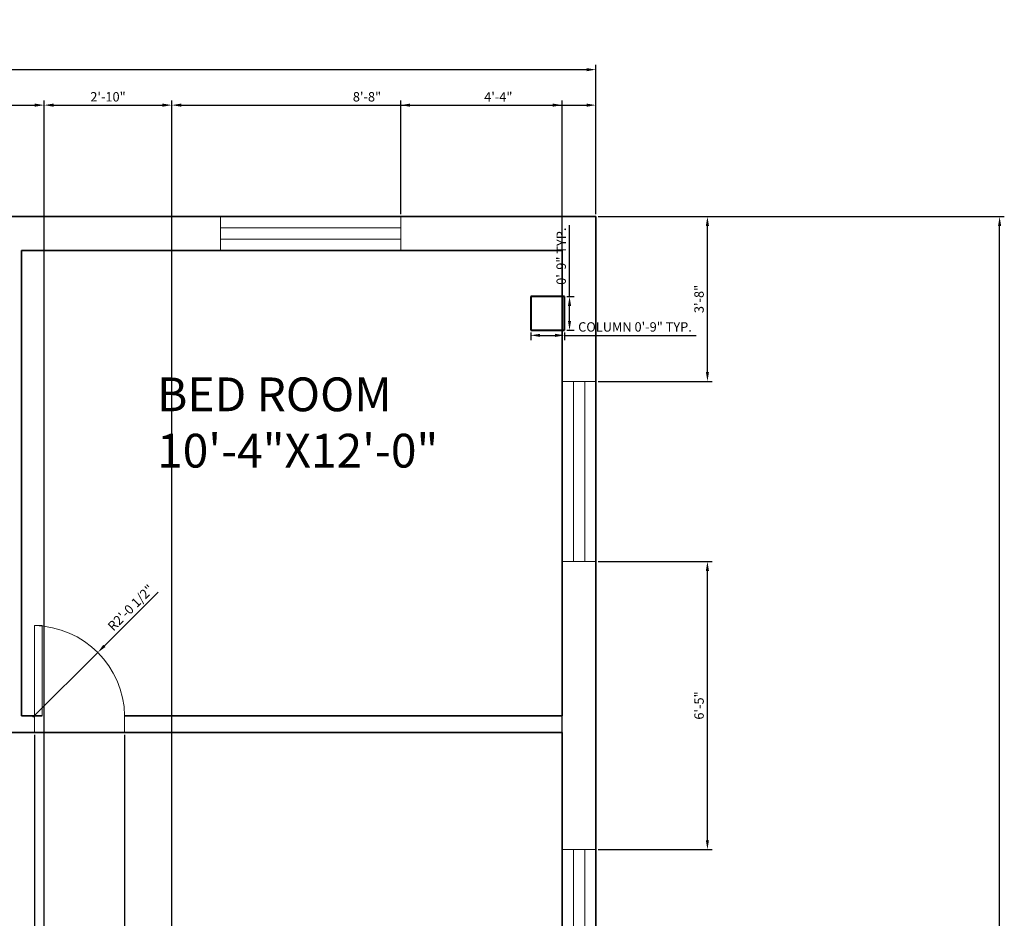
# Model space of a CAD drawing. Units: millimetres. Extents: x 2124 to 2653, y 1244 to 1836.
# Tile 4 of 4: x 2390 to 2653, y 1597 to 1836. Entities that reach past the tile are written whole.
import ezdxf

# ---------------------------------------------------------------- set-up
doc = ezdxf.new("R2010")
doc.units = ezdxf.units.MM
for name, color, linetype, lineweight in [('A-ANNO-DIMS', 2, 'Continuous', 18), ('A-AREA-IDEN', 7, 'Continuous', 18), ('A-COLS', 1, 'Continuous', 40), ('A-DOOR', 3, 'Continuous', 18), ('A-GLAZ', 4, 'Continuous', 18), ('A-WALL', 7, 'Continuous', 35)]:
    doc.layers.add(name, color=color, linetype=linetype, lineweight=lineweight)
doc.styles.get("Standard").update_dxf_attribs({"font": 'arial.ttf'})
doc.dimstyles.new('ISO-25', dxfattribs={"dimtxt": 2.5, "dimasz": 2.5, "dimexe": 1.25, "dimexo": 0.625, "dimtad": 1, "dimdec": 0, "dimlunit": 3, "dimtxsty": 'Standard', "dimcen": 2.5, "dimadec": 0, "dimazin": 0, "dimtfac": 1, "dimtdec": 0, "dimtmove": 0, "dimatfit": 3, "dimfxl": 1, "dimarcsym": 0})

# ---------------------------------------------------------------- blocks, each defined once
blk = doc.blocks.new('*D8')
at = {"layer": 'A-ANNO-DIMS', "color": 0, "lineweight": -2, "transparency": 16777216}
for p, q in [((2159.76, 1784.37), (2159.76, 1824.15)), ((2162.26, 1822.9), (2541.26, 1822.9)), ((2543.76, 1784.37), (2543.76, 1824.15))]:
    blk.add_line(p, q, dxfattribs=at)
at = {"layer": 'A-ANNO-DIMS', "color": 0, "transparency": 16777216}
for points in [[(2162.26, 1823.31), (2162.26, 1822.48), (2159.76, 1822.9)], [(2541.26, 1823.31), (2541.26, 1822.48), (2543.76, 1822.9)]]:
    blk.add_solid(points, dxfattribs=at)
at = {"layer": 'Defpoints', "color": 0, "transparency": 16777216}
for p in [(2543.76, 1822.9), (2159.76, 1783.74), (2543.76, 1783.74)]:
    blk.add_point(p, dxfattribs=at)
at = {"layer": 'A-ANNO-DIMS', "color": 0, "transparency": 16777216, "insert": (2351.76, 1829.59), "char_height": 2.5, "attachment_point": 5}
blk.add_mtext("{\\fCambria|b0|i0|c0|p18;\\H4.8x;32'}", dxfattribs=at)
blk = doc.blocks.new('*D9')
at = {"layer": 'A-ANNO-DIMS', "color": 0, "lineweight": -2, "transparency": 16777216}
for p, q in [((2544.38, 1783.74), (2652.54, 1783.74)), ((2651.29, 1289.47), (2651.29, 1781.24)), ((2544.38, 1286.97), (2652.54, 1286.97))]:
    blk.add_line(p, q, dxfattribs=at)
at = {"layer": 'A-ANNO-DIMS', "color": 0, "transparency": 16777216}
for points in [[(2650.87, 1781.24), (2651.71, 1781.24), (2651.29, 1783.74)], [(2650.87, 1289.47), (2651.71, 1289.47), (2651.29, 1286.97)]]:
    blk.add_solid(points, dxfattribs=at)
at = {"layer": 'Defpoints', "color": 0, "transparency": 16777216}
for p in [(2543.76, 1783.74), (2651.29, 1783.74), (2543.76, 1286.97)]:
    blk.add_point(p, dxfattribs=at)
at = {"layer": 'A-ANNO-DIMS', "color": 0, "transparency": 16777216, "insert": (2644.38, 1535.36), "char_height": 2.5, "width": 21.1968, "attachment_point": 5, "rotation": 90}
blk.add_mtext('{\\fCambria|b0|i0|c0|p18;\\H4.8x;45\'-0"}', dxfattribs=at)
blk = doc.blocks.new('WINDOW-4FT')
for p, q in [((48, 9), (0, 9)), ((0, 9), (0, 0)), ((48, 0), (48, 9)), ((48, 6), (0, 6)), ((48, 3), (0, 3)), ((0, 0), (48, 0))]:
    blk.add_line(p, q)
blk = doc.blocks.new('WINDOW-2FT')
for p, q in [((9, 24), (0, 24)), ((0, 24), (0, 0)), ((3, 0), (3, 24)), ((6, 0), (6, 24)), ((9, 0), (9, 24)), ((0, 0), (9, 0))]:
    blk.add_line(p, q)
blk = doc.blocks.new('COLUMN-9IN-SQ')
for p, q in [((9, 9), (0, 9)), ((0, 9), (0, 0)), ((9, 0), (9, 9)), ((0, 0), (9, 0))]:
    blk.add_line(p, q)
blk = doc.blocks.new('*D16')
at = {"layer": 'A-ANNO-DIMS', "color": 0, "lineweight": -2, "transparency": 16777216}
for p, q in [((2526.38, 1752.82), (2526.38, 1750.85)), ((2528.88, 1752.1), (2532.88, 1752.1)), ((2535.38, 1752.82), (2535.38, 1750.85)), ((2535.38, 1752.1), (2570.44, 1752.1))]:
    blk.add_line(p, q, dxfattribs=at)
at = {"layer": 'A-ANNO-DIMS', "color": 0, "transparency": 16777216}
for points in [[(2528.88, 1752.51), (2528.88, 1751.68), (2526.38, 1752.1)], [(2532.88, 1752.51), (2532.88, 1751.68), (2535.38, 1752.1)]]:
    blk.add_solid(points, dxfattribs=at)
at = {"layer": 'Defpoints', "color": 0, "transparency": 16777216}
for p in [(2526.38, 1753.45), (2535.38, 1753.45), (2535.38, 1752.1)]:
    blk.add_point(p, dxfattribs=at)
at = {"layer": 'A-ANNO-DIMS', "color": 0, "transparency": 16777216, "insert": (2554.16, 1754.02), "char_height": 2.5, "attachment_point": 5}
blk.add_mtext('COLUMN 0\'-9" TYP.', dxfattribs=at)
blk = doc.blocks.new('*D17')
at = {"layer": 'A-ANNO-DIMS', "color": 0, "lineweight": -2, "transparency": 16777216}
for p, q in [((2536.73, 1762.45), (2536.73, 1781.44)), ((2536, 1762.45), (2537.98, 1762.45)), ((2536.73, 1755.95), (2536.73, 1759.95)), ((2536, 1753.45), (2537.98, 1753.45))]:
    blk.add_line(p, q, dxfattribs=at)
at = {"layer": 'A-ANNO-DIMS', "color": 0, "transparency": 16777216}
for points in [[(2536.31, 1759.95), (2537.14, 1759.95), (2536.73, 1762.45)], [(2536.31, 1755.95), (2537.14, 1755.95), (2536.73, 1753.45)]]:
    blk.add_solid(points, dxfattribs=at)
at = {"layer": 'Defpoints', "color": 0, "transparency": 16777216}
for p in [(2535.38, 1762.45), (2536.73, 1762.45), (2535.38, 1753.45)]:
    blk.add_point(p, dxfattribs=at)
at = {"layer": 'A-ANNO-DIMS', "color": 0, "transparency": 16777216, "insert": (2534.83, 1773.19), "char_height": 2.5, "attachment_point": 5, "rotation": 90}
blk.add_mtext('0\'-9" TYP.', dxfattribs=at)
blk = doc.blocks.new('*D22')
at = {"layer": 'A-ANNO-DIMS', "color": 0, "lineweight": -2, "transparency": 16777216}
for p, q in [((2491.76, 1784.37), (2491.76, 1814.69)), ((2494.26, 1813.44), (2541.26, 1813.44)), ((2543.76, 1784.37), (2543.76, 1814.69))]:
    blk.add_line(p, q, dxfattribs=at)
at = {"layer": 'A-ANNO-DIMS', "color": 0, "transparency": 16777216}
for points in [[(2494.26, 1813.86), (2494.26, 1813.02), (2491.76, 1813.44)], [(2541.26, 1813.86), (2541.26, 1813.02), (2543.76, 1813.44)]]:
    blk.add_solid(points, dxfattribs=at)
at = {"layer": 'Defpoints', "color": 0, "transparency": 16777216}
for p in [(2543.76, 1813.44), (2491.76, 1783.74), (2543.76, 1783.74)]:
    blk.add_point(p, dxfattribs=at)
at = {"layer": 'A-ANNO-DIMS', "color": 0, "transparency": 16777216, "insert": (2517.76, 1815.32), "char_height": 2.5, "attachment_point": 5}
blk.add_mtext('4\'-4"', dxfattribs=at)
blk = doc.blocks.new('*D24')
at = {"layer": 'A-ANNO-DIMS', "color": 0, "lineweight": -2, "transparency": 16777216}
for p, q in [((2544.38, 1783.74), (2574.71, 1783.74)), ((2573.46, 1742.34), (2573.46, 1781.24)), ((2544.38, 1739.84), (2574.71, 1739.84))]:
    blk.add_line(p, q, dxfattribs=at)
at = {"layer": 'A-ANNO-DIMS', "color": 0, "transparency": 16777216}
for points in [[(2573.04, 1781.24), (2573.87, 1781.24), (2573.46, 1783.74)], [(2573.04, 1742.34), (2573.87, 1742.34), (2573.46, 1739.84)]]:
    blk.add_solid(points, dxfattribs=at)
at = {"layer": 'Defpoints', "color": 0, "transparency": 16777216}
for p in [(2543.76, 1783.74), (2573.46, 1783.74), (2543.76, 1739.84)]:
    blk.add_point(p, dxfattribs=at)
at = {"layer": 'A-ANNO-DIMS', "color": 0, "transparency": 16777216, "insert": (2571.55, 1761.79), "char_height": 2.5, "attachment_point": 5, "rotation": 90}
blk.add_mtext('3\'-8"', dxfattribs=at)
blk = doc.blocks.new('*D25')
at = {"layer": 'A-ANNO-DIMS', "color": 0, "lineweight": -2, "transparency": 16777216}
for p, q in [((2544.38, 1691.84), (2574.71, 1691.84)), ((2573.46, 1617.57), (2573.46, 1689.34)), ((2544.38, 1615.07), (2574.71, 1615.07))]:
    blk.add_line(p, q, dxfattribs=at)
at = {"layer": 'A-ANNO-DIMS', "color": 0, "transparency": 16777216}
for points in [[(2573.04, 1689.34), (2573.87, 1689.34), (2573.46, 1691.84)], [(2573.04, 1617.57), (2573.87, 1617.57), (2573.46, 1615.07)]]:
    blk.add_solid(points, dxfattribs=at)
at = {"layer": 'Defpoints', "color": 0, "transparency": 16777216}
for p in [(2543.76, 1691.84), (2573.46, 1691.84), (2543.76, 1615.07)]:
    blk.add_point(p, dxfattribs=at)
at = {"layer": 'A-ANNO-DIMS', "color": 0, "transparency": 16777216, "insert": (2571.55, 1653.46), "char_height": 2.5, "attachment_point": 5, "rotation": 90}
blk.add_mtext('6\'-5"', dxfattribs=at)
blk = doc.blocks.new('*D43')
at = {"layer": 'A-ANNO-DIMS', "color": 0, "lineweight": -2, "transparency": 16777216}
for p, q in [((2383.02, 1645.62), (2383.02, 1256.02)), ((2394.21, 1645.62), (2394.21, 1256.02)), ((2385.52, 1257.27), (2391.71, 1257.27))]:
    blk.add_line(p, q, dxfattribs=at)
at = {"layer": 'A-ANNO-DIMS', "color": 0, "transparency": 16777216}
for points in [[(2385.52, 1257.69), (2385.52, 1256.86), (2383.02, 1257.27)], [(2391.71, 1257.69), (2391.71, 1256.86), (2394.21, 1257.27)]]:
    blk.add_solid(points, dxfattribs=at)
at = {"layer": 'Defpoints', "color": 0, "transparency": 16777216}
for p in [(2383.02, 1646.24), (2394.21, 1646.24), (2394.21, 1257.27)]:
    blk.add_point(p, dxfattribs=at)
at = {"layer": 'A-ANNO-DIMS', "color": 0, "transparency": 16777216, "insert": (2388.62, 1259.18), "char_height": 2.5, "attachment_point": 5}
blk.add_mtext('0\'-11"', dxfattribs=at)
blk = doc.blocks.new('*D44')
at = {"layer": 'A-ANNO-DIMS', "color": 0, "lineweight": -2, "transparency": 16777216}
for p, q in [((2394.21, 1645.62), (2394.21, 1256.02)), ((2418.21, 1645.62), (2418.21, 1256.02)), ((2396.71, 1257.27), (2415.71, 1257.27))]:
    blk.add_line(p, q, dxfattribs=at)
at = {"layer": 'A-ANNO-DIMS', "color": 0, "transparency": 16777216}
for points in [[(2396.71, 1257.69), (2396.71, 1256.86), (2394.21, 1257.27)], [(2415.71, 1257.69), (2415.71, 1256.86), (2418.21, 1257.27)]]:
    blk.add_solid(points, dxfattribs=at)
at = {"layer": 'Defpoints', "color": 0, "transparency": 16777216}
for p in [(2394.21, 1646.24), (2418.21, 1646.24), (2418.21, 1257.27)]:
    blk.add_point(p, dxfattribs=at)
at = {"layer": 'A-ANNO-DIMS', "color": 0, "transparency": 16777216, "insert": (2406.21, 1259.18), "char_height": 2.5, "attachment_point": 5}
blk.add_mtext('2\'-0"', dxfattribs=at)
blk = doc.blocks.new('*D45')
at = {"layer": 'A-ANNO-DIMS', "color": 0, "lineweight": -2, "transparency": 16777216}
for p, q in [((2418.21, 1645.62), (2418.21, 1256.02)), ((2534.76, 1645.62), (2534.76, 1256.02)), ((2420.71, 1257.27), (2532.26, 1257.27))]:
    blk.add_line(p, q, dxfattribs=at)
at = {"layer": 'A-ANNO-DIMS', "color": 0, "transparency": 16777216}
for points in [[(2420.71, 1257.69), (2420.71, 1256.86), (2418.21, 1257.27)], [(2532.26, 1257.69), (2532.26, 1256.86), (2534.76, 1257.27)]]:
    blk.add_solid(points, dxfattribs=at)
at = {"layer": 'Defpoints', "color": 0, "transparency": 16777216}
for p in [(2418.21, 1646.24), (2534.76, 1646.24), (2534.76, 1257.27)]:
    blk.add_point(p, dxfattribs=at)
at = {"layer": 'A-ANNO-DIMS', "color": 0, "transparency": 16777216, "insert": (2476.48, 1259.19), "char_height": 2.5, "attachment_point": 5}
blk.add_mtext('9\'-8 1/2"', dxfattribs=at)
blk = doc.blocks.new('*D47')
at = {"layer": 'A-ANNO-DIMS', "color": 0, "lineweight": -2, "transparency": 16777216}
for p, q in [((2365.24, 1448.87), (2365.24, 1814.69)), ((2367.74, 1813.44), (2394.29, 1813.44)), ((2396.79, 1448.87), (2396.79, 1814.69))]:
    blk.add_line(p, q, dxfattribs=at)
at = {"layer": 'A-ANNO-DIMS', "color": 0, "transparency": 16777216}
for points in [[(2367.74, 1813.86), (2367.74, 1813.02), (2365.24, 1813.44)], [(2394.29, 1813.86), (2394.29, 1813.02), (2396.79, 1813.44)]]:
    blk.add_solid(points, dxfattribs=at)
at = {"layer": 'Defpoints', "color": 0, "transparency": 16777216}
for p in [(2396.79, 1813.44), (2365.24, 1448.24), (2396.79, 1448.24)]:
    blk.add_point(p, dxfattribs=at)
at = {"layer": 'A-ANNO-DIMS', "color": 0, "transparency": 16777216, "insert": (2381.02, 1815.36), "char_height": 2.5, "attachment_point": 5}
blk.add_mtext('2\'-7 1/2"', dxfattribs=at)
blk = doc.blocks.new('*D48')
at = {"layer": 'A-ANNO-DIMS', "color": 0, "lineweight": -2, "transparency": 16777216}
for p, q in [((2396.79, 1448.87), (2396.79, 1814.69)), ((2399.29, 1813.44), (2428.29, 1813.44)), ((2430.79, 1448.87), (2430.79, 1814.69))]:
    blk.add_line(p, q, dxfattribs=at)
at = {"layer": 'A-ANNO-DIMS', "color": 0, "transparency": 16777216}
for points in [[(2399.29, 1813.86), (2399.29, 1813.02), (2396.79, 1813.44)], [(2428.29, 1813.86), (2428.29, 1813.02), (2430.79, 1813.44)]]:
    blk.add_solid(points, dxfattribs=at)
at = {"layer": 'Defpoints', "color": 0, "transparency": 16777216}
for p in [(2430.79, 1813.44), (2396.79, 1448.24), (2430.79, 1448.24)]:
    blk.add_point(p, dxfattribs=at)
at = {"layer": 'A-ANNO-DIMS', "color": 0, "transparency": 16777216, "insert": (2413.79, 1815.34), "char_height": 2.5, "attachment_point": 5}
blk.add_mtext('2\'-10"', dxfattribs=at)
blk = doc.blocks.new('*D49')
at = {"layer": 'A-ANNO-DIMS', "color": 0, "lineweight": -2, "transparency": 16777216}
for p, q in [((2430.79, 1448.87), (2430.79, 1814.69)), ((2433.29, 1813.44), (2532.26, 1813.44)), ((2534.76, 1448.87), (2534.76, 1814.69))]:
    blk.add_line(p, q, dxfattribs=at)
at = {"layer": 'A-ANNO-DIMS', "color": 0, "transparency": 16777216}
for points in [[(2433.29, 1813.86), (2433.29, 1813.02), (2430.79, 1813.44)], [(2532.26, 1813.86), (2532.26, 1813.02), (2534.76, 1813.44)]]:
    blk.add_solid(points, dxfattribs=at)
at = {"layer": 'Defpoints', "color": 0, "transparency": 16777216}
for p in [(2534.76, 1813.44), (2430.79, 1448.24), (2534.76, 1448.24)]:
    blk.add_point(p, dxfattribs=at)
at = {"layer": 'A-ANNO-DIMS', "color": 0, "transparency": 16777216, "insert": (2482.77, 1815.34), "char_height": 2.5, "attachment_point": 5}
blk.add_mtext('8\'-8"', dxfattribs=at)
blk = doc.blocks.new('*D61')
at = {"layer": 'A-ANNO-DIMS', "color": 0, "lineweight": -2, "transparency": 16777216}
for p, q in [((2427.12, 1683.65), (2412.83, 1669.35)), ((2393.78, 1650.31), (2411.06, 1667.59))]:
    blk.add_line(p, q, dxfattribs=at)
at = {"layer": 'A-ANNO-DIMS', "color": 0, "transparency": 16777216}
blk.add_solid([(2412.53, 1669.65), (2413.12, 1669.06), (2411.06, 1667.59)], dxfattribs=at)
at = {"layer": 'Defpoints', "color": 0, "transparency": 16777216}
for p in [(2411.06, 1667.59), (2393.78, 1650.31)]:
    blk.add_point(p, dxfattribs=at)
at = {"layer": 'A-ANNO-DIMS', "color": 0, "transparency": 16777216, "insert": (2420.07, 1679.31), "char_height": 2.5, "attachment_point": 5, "rotation": 44.9997}
blk.add_mtext('R2\'-0 1/2"', dxfattribs=at)

msp = doc.modelspace()

# ---------------------------------------------------------------- linework, layer by layer
at = {"layer": 'A-DOOR'}
for p, q in [((2394.21, 1650.74), (2394.21, 1674.74)), ((2394.21, 1674.74), (2396.21, 1674.74)), ((2396.21, 1674.74), (2396.21, 1650.74)), ((2394.21, 1646.24), (2394.21, 1650.74)), ((2418.21, 1646.24), (2418.21, 1650.74))]:
    msp.add_line(p, q, dxfattribs=at)
msp.add_arc((2393.78, 1650.31), 24.44, 1.016, 88.984, dxfattribs=at)
at = {"layer": 'A-GLAZ'}
msp.add_line((2473.58, 1777.74), (2471.58, 1777.74), dxfattribs=at)
at = {"layer": 'A-WALL'}
for p, q in [((2543.76, 1783.74), (2159.76, 1783.74)), ((2543.76, 1286.97), (2543.76, 1783.74)), ((2534.76, 1774.74), (2390.76, 1774.74)), ((2390.76, 1650.74), (2390.76, 1774.74)), ((2534.76, 1650.74), (2534.76, 1774.74)), ((2396.21, 1650.74), (2390.76, 1650.74)), ((2534.76, 1650.74), (2418.21, 1650.74)), ((2534.76, 1646.24), (2383.02, 1646.24)), ((2534.76, 1448.24), (2534.76, 1646.24))]:
    msp.add_line(p, q, dxfattribs=at)

# ---------------------------------------------------------------- block references
at = {"layer": 'A-COLS'}
msp.add_blockref('COLUMN-9IN-SQ', (2526.38, 1753.45), dxfattribs=at)
at = {"layer": 'A-GLAZ'}
for p, rotation in [((2491.76, 1783.74), 180), ((2491.76, 1783.74), 180), ((2534.76, 1739.84), 270.0000000000007)]:
    msp.add_blockref('WINDOW-4FT', p, dxfattribs=dict(at, rotation=rotation))
msp.add_blockref('WINDOW-2FT', (2534.76, 1591.07), dxfattribs=at)

# ---------------------------------------------------------------- texts
at = {"layer": 'A-AREA-IDEN', "insert": (2426.87, 1740.87), "char_height": 9, "attachment_point": 1}
msp.add_mtext_dynamic_manual_height_columns('{\\fCambria|b0|i0|c0|p18;BED ROOM\\P10\'-4"X12\'-0"}', width=93.0425, gutter_width=12.5, heights=[0], dxfattribs=at)

# ---------------------------------------------------------------- dimensions: what is measured, and where the dimension line sits
at = {"layer": 'A-ANNO-DIMS'}
for base, p1, p2, text, override, picture, middle in [((2543.76, 1822.9), (2159.76, 1783.74), (2543.76, 1783.74), '{\\fCambria|b0|i0|c0|p18;\\H4.8x;<>}', {"dimclrd": 0, "dimclre": 0, "dimclrt": 0}, '*D8', (2351.76, 1829.59)), ((2535.38, 1752.1), (2526.38, 1753.45), (2535.38, 1753.45), 'COLUMN <> TYP.', {"dimdec": 1, "dimlfac": 1, "dimrnd": 0, "dimzin": 1, "dimdsep": 46, "dimlunit": 4, "dimfrac": 2}, '*D16', (2554.16, 1754.02))]:
    dim = msp.add_linear_dim(base=base, p1=p1, p2=p2, text=text, dimstyle='ISO-25', override=override, dxfattribs=at)
    dim.commit()
    dim.dimension.update_dxf_attribs({"geometry": picture, "text_midpoint": middle})
for base, p1, p2, picture, middle in [((2396.7929, 1813.4406), (2365.2427, 1448.2406), (2396.7929, 1448.2406), '*D47', (2381.0178, 1815.3582)), ((2430.79, 1813.44), (2396.79, 1448.24), (2430.79, 1448.24), '*D48', (2413.79, 1815.34)), ((2534.76, 1813.44), (2430.79, 1448.24), (2534.76, 1448.24), '*D49', (2482.77, 1815.34)), ((2543.76, 1813.44), (2491.76, 1783.74), (2543.76, 1783.74), '*D22', (2517.76, 1815.32)), ((2394.21, 1257.27), (2383.02, 1646.24), (2394.21, 1646.24), '*D43', (2388.62, 1259.18)), ((2418.21, 1257.27), (2394.21, 1646.24), (2418.21, 1646.24), '*D44', (2406.21, 1259.18)), ((2534.7564, 1257.2741), (2418.2124, 1646.2406), (2534.7564, 1646.2406), '*D45', (2476.4844, 1259.1917))]:
    dim = msp.add_linear_dim(base=base, p1=p1, p2=p2, dimstyle='ISO-25', override={"dimdec": 1, "dimlfac": 1, "dimrnd": 0, "dimzin": 1, "dimdsep": 46, "dimlunit": 4, "dimfrac": 2}, dxfattribs=at)
    dim.commit()
    dim.dimension.update_dxf_attribs({"geometry": picture, "text_midpoint": middle})
for base, p1, p2, text, override, picture, middle in [((2651.29, 1783.74), (2543.76, 1286.97), (2543.76, 1783.74), '{\\fCambria|b0|i0|c0|p18;\\H4.8x;45\'-0"}', {"dimclrd": 0, "dimclre": 0, "dimclrt": 0}, '*D9', (2644.38, 1535.36)), ((2536.73, 1762.45), (2535.38, 1753.45), (2535.38, 1762.45), '<> TYP.', {"dimdec": 1, "dimlfac": 1, "dimrnd": 0, "dimzin": 1, "dimdsep": 46, "dimlunit": 4, "dimfrac": 2}, '*D17', (2534.83, 1773.19))]:
    dim = msp.add_linear_dim(base=base, p1=p1, p2=p2, angle=90, text=text, dimstyle='ISO-25', override=override, dxfattribs=at)
    dim.commit()
    dim.dimension.update_dxf_attribs({"geometry": picture, "text_midpoint": middle})
for base, p1, p2, picture, middle in [((2573.46, 1783.74), (2543.76, 1739.84), (2543.76, 1783.74), '*D24', (2571.55, 1761.79)), ((2573.46, 1691.84), (2543.76, 1615.07), (2543.76, 1691.84), '*D25', (2571.55, 1653.46))]:
    dim = msp.add_linear_dim(base=base, p1=p1, p2=p2, angle=90, dimstyle='ISO-25', override={"dimdec": 1, "dimlfac": 1, "dimrnd": 0, "dimzin": 1, "dimdsep": 46, "dimlunit": 4, "dimfrac": 2}, dxfattribs=at)
    dim.commit()
    dim.dimension.update_dxf_attribs({"geometry": picture, "text_midpoint": middle})
dim = msp.add_radius_dim(center=(2393.78, 1650.31), mpoint=(2411.06, 1667.59), dimstyle='ISO-25', override={"dimdec": 1, "dimlfac": 1, "dimrnd": 0, "dimzin": 1, "dimdsep": 46, "dimlunit": 4, "dimfrac": 2}, dxfattribs=at)
dim.commit()
dim.dimension.update_dxf_attribs({"geometry": '*D61', "text_midpoint": (2421.43, 1677.95), "dimtype": 164})

doc.saveas('drawing.dxf')
